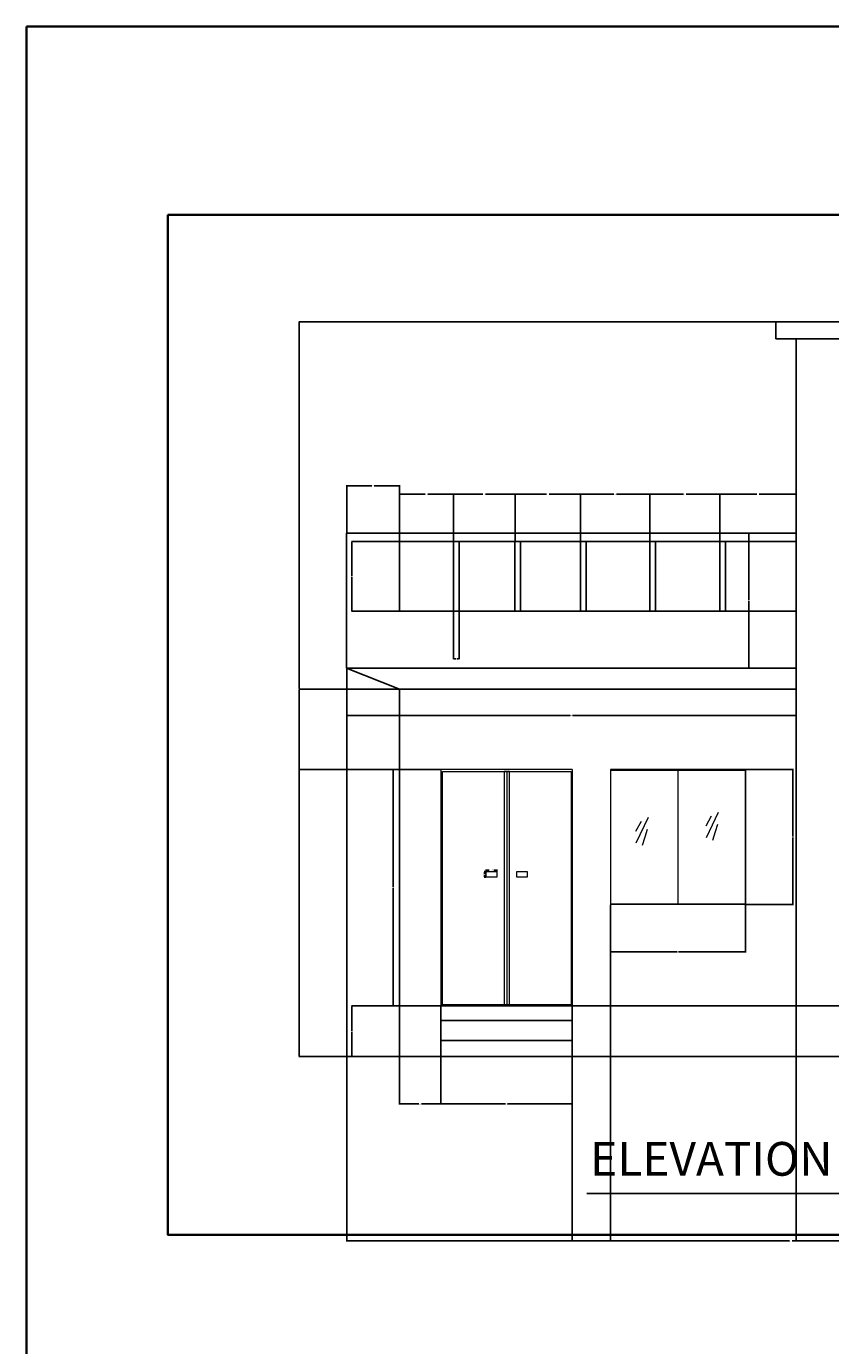
# Model space of a CAD drawing. Units: inches. Extents: x 1976 to 2558, y -977 to 2909.
# Tile 7 of 8: x 1976 to 2262, y 2441 to 2909. Entities that reach past the tile are written whole.
import ezdxf

# ---------------------------------------------------------------- set-up
doc = ezdxf.new("R2010")
doc.units = ezdxf.units.IN
for name, color, linetype, lineweight in [('A-ANNO-DIMS', 2, 'Continuous', 18), ('A-ANNO-TEXT', 7, 'Continuous', 25), ('A-ANNO-TTLB', 7, 'Continuous', 35), ('A-ELEV', 7, 'Continuous', 25), ('A-ELEV-DOOR', 3, 'Continuous', 18), ('A-ELEV-GLAZ', 4, 'Continuous', 18)]:
    doc.layers.add(name, color=color, linetype=linetype, lineweight=lineweight)
doc.styles.get("Standard").update_dxf_attribs({"font": 'arial.ttf'})
doc.dimstyles.get("Standard").update_dxf_attribs({"dimtxt": 0.18, "dimasz": 0.18, "dimexe": 0.18, "dimexo": 0.0625, "dimgap": 0.09, "dimtad": 0, "dimtih": 1, "dimtoh": 1, "dimdec": 4, "dimzin": 0, "dimdsep": 46, "dimtxsty": 'Standard', "dimcen": 0.09, "dimadec": 0, "dimazin": 0, "dimtfac": 1, "dimtdec": 4, "dimtofl": 0, "dimtmove": 0, "dimatfit": 3, "dimfxl": 1, "dimtolj": 1, "dimtzin": 0, "dimarcsym": 0})

# ---------------------------------------------------------------- blocks, each defined once
blk = doc.blocks.new('GLASS-REFLECTION')
for p, q in [((4.44, 9.97), (0.12, 0.93)), ((1.95, 8.6), (0, 5.03)), ((4.15, 5.7), (3.32, 3.04)), ((3.32, 3.04), (2.37, 0))]:
    blk.add_line(p, q)
blk = doc.blocks.new('DOOR-PULL-ELEV')
blk.add_lwpolyline([(0, 2.02), (3.74, 2.02), (3.74, 0), (0, 0)], close=True)
blk = doc.blocks.new('*D21')
at = {"layer": 'A-ANNO-DIMS', "color": 0, "lineweight": -2, "transparency": 16777216}
for p, q in [((2139.28, 2609.02), (2139.28, 2609.7)), ((2139.46, 2609.52), (2140.35, 2609.52)), ((2142.84, 2609.52), (2141.96, 2609.52)), ((2143.02, 2609.02), (2143.02, 2609.7))]:
    blk.add_line(p, q, dxfattribs=at)
at = {"layer": 'A-ANNO-DIMS', "color": 0, "transparency": 16777216}
for points in [[(2139.46, 2609.55), (2139.46, 2609.49), (2139.28, 2609.52)], [(2142.84, 2609.55), (2142.84, 2609.49), (2143.02, 2609.52)]]:
    blk.add_solid(points, dxfattribs=at)
at = {"layer": 'Defpoints', "color": 0, "transparency": 16777216}
for p in [(2139.28, 2608.96), (2143.02, 2609.52), (2143.02, 2608.96)]:
    blk.add_point(p, dxfattribs=at)
at = {"layer": 'A-ANNO-DIMS', "color": 0, "transparency": 16777216, "insert": (2141.15, 2609.52), "char_height": 0.18, "attachment_point": 5}
blk.add_mtext('\\A1;PULL 4 TYP.', dxfattribs=at)
blk = doc.blocks.new('*D22')
at = {"layer": 'A-ANNO-DIMS', "color": 0, "lineweight": -2, "transparency": 16777216}
for p, q in [((2139.22, 2608.96), (2138.54, 2608.96)), ((2139.22, 2606.94), (2138.54, 2606.94)), ((2138.72, 2608.78), (2138.72, 2608.13)), ((2138.72, 2607.12), (2138.72, 2607.77))]:
    blk.add_line(p, q, dxfattribs=at)
at = {"layer": 'A-ANNO-DIMS', "color": 0, "transparency": 16777216}
for points in [[(2138.69, 2608.78), (2138.75, 2608.78), (2138.72, 2608.96)], [(2138.69, 2607.12), (2138.75, 2607.12), (2138.72, 2606.94)]]:
    blk.add_solid(points, dxfattribs=at)
at = {"layer": 'Defpoints', "color": 0, "transparency": 16777216}
for p in [(2138.72, 2608.96), (2139.28, 2608.96), (2139.28, 2606.94)]:
    blk.add_point(p, dxfattribs=at)
at = {"layer": 'A-ANNO-DIMS', "color": 0, "transparency": 16777216, "insert": (2138.72, 2607.95), "char_height": 0.18, "attachment_point": 5}
blk.add_mtext('\\A1;2 TYP.', dxfattribs=at)
blk = doc.blocks.new('*D51')
at = {"layer": 'A-ANNO-DIMS', "color": 0, "lineweight": -2, "transparency": 16777216}
for p, q in [((2089.7, 2681.2), (2089.7, 2477.53)), ((2405.44, 2543.2), (2405.44, 2477.53)), ((2089.88, 2477.71), (2247.1, 2477.71)), ((2405.26, 2477.71), (2248.03, 2477.71))]:
    blk.add_line(p, q, dxfattribs=at)
at = {"layer": 'A-ANNO-DIMS', "color": 0, "transparency": 16777216}
for points in [[(2089.88, 2477.74), (2089.88, 2477.68), (2089.7, 2477.71)], [(2405.26, 2477.74), (2405.26, 2477.68), (2405.44, 2477.71)]]:
    blk.add_solid(points, dxfattribs=at)
at = {"layer": 'Defpoints', "color": 0, "transparency": 16777216}
for p in [(2089.7, 2681.26), (2405.44, 2543.26), (2405.44, 2477.71)]:
    blk.add_point(p, dxfattribs=at)
at = {"layer": 'A-ANNO-DIMS', "color": 0, "transparency": 16777216, "insert": (2247.57, 2477.71), "char_height": 0.18, "attachment_point": 5}
blk.add_mtext('\\A1;315.74', dxfattribs=at)
blk = doc.blocks.new('*D52')
at = {"layer": 'A-ANNO-DIMS', "color": 0, "lineweight": -2, "transparency": 16777216}
for p, q in [((2242.18, 2804.36), (2072.67, 2804.36)), ((2072.85, 2804.18), (2072.85, 2673.99)), ((2072.85, 2543.44), (2072.85, 2673.63)), ((2108.38, 2543.26), (2072.67, 2543.26))]:
    blk.add_line(p, q, dxfattribs=at)
at = {"layer": 'A-ANNO-DIMS', "color": 0, "transparency": 16777216}
for points in [[(2072.82, 2804.18), (2072.88, 2804.18), (2072.85, 2804.36)], [(2072.82, 2543.44), (2072.88, 2543.44), (2072.85, 2543.26)]]:
    blk.add_solid(points, dxfattribs=at)
at = {"layer": 'Defpoints', "color": 0, "transparency": 16777216}
for p in [(2072.85, 2804.36), (2242.24, 2804.36), (2108.44, 2543.26)]:
    blk.add_point(p, dxfattribs=at)
at = {"layer": 'A-ANNO-DIMS', "color": 0, "transparency": 16777216, "insert": (2072.85, 2673.81), "char_height": 0.18, "attachment_point": 5}
blk.add_mtext('\\A1;261.1', dxfattribs=at)
blk = doc.blocks.new('*D53')
at = {"layer": 'A-ANNO-DIMS', "color": 0, "lineweight": -2, "transparency": 16777216}
for p, q in [((2108.38, 2561.26), (2091.41, 2561.26)), ((2091.59, 2561.08), (2091.59, 2552.44)), ((2091.59, 2543.44), (2091.59, 2552.08)), ((2108.38, 2543.26), (2091.41, 2543.26))]:
    blk.add_line(p, q, dxfattribs=at)
at = {"layer": 'A-ANNO-DIMS', "color": 0, "transparency": 16777216}
for points in [[(2091.56, 2561.08), (2091.62, 2561.08), (2091.59, 2561.26)], [(2091.56, 2543.44), (2091.62, 2543.44), (2091.59, 2543.26)]]:
    blk.add_solid(points, dxfattribs=at)
at = {"layer": 'Defpoints', "color": 0, "transparency": 16777216}
for p in [(2091.59, 2561.26), (2108.44, 2561.26), (2108.44, 2543.26)]:
    blk.add_point(p, dxfattribs=at)
at = {"layer": 'A-ANNO-DIMS', "color": 0, "transparency": 16777216, "insert": (2091.59, 2552.26), "char_height": 0.18, "attachment_point": 5}
blk.add_mtext('\\A1;18', dxfattribs=at)
blk = doc.blocks.new('*D54')
at = {"layer": 'A-ANNO-DIMS', "color": 0, "lineweight": -2, "transparency": 16777216}
for p, q in [((2123.06, 2645.26), (2106.09, 2645.26)), ((2106.27, 2645.08), (2106.27, 2603.44)), ((2106.27, 2561.44), (2106.27, 2603.08)), ((2123.06, 2561.26), (2106.09, 2561.26))]:
    blk.add_line(p, q, dxfattribs=at)
at = {"layer": 'A-ANNO-DIMS', "color": 0, "transparency": 16777216}
for points in [[(2106.24, 2645.08), (2106.3, 2645.08), (2106.27, 2645.26)], [(2106.24, 2561.44), (2106.3, 2561.44), (2106.27, 2561.26)]]:
    blk.add_solid(points, dxfattribs=at)
at = {"layer": 'Defpoints', "color": 0, "transparency": 16777216}
for p in [(2106.27, 2645.26), (2123.12, 2645.26), (2123.12, 2561.26)]:
    blk.add_point(p, dxfattribs=at)
at = {"layer": 'A-ANNO-DIMS', "color": 0, "transparency": 16777216, "insert": (2106.27, 2603.26), "char_height": 0.18, "attachment_point": 5}
blk.add_mtext('\\A1;84', dxfattribs=at)
blk = doc.blocks.new('*D55')
at = {"layer": 'A-ANNO-DIMS', "color": 0, "lineweight": -2, "transparency": 16777216}
for p, q in [((2108.38, 2673.8), (2072.67, 2673.8)), ((2072.85, 2673.62), (2072.85, 2659.71)), ((2072.85, 2645.44), (2072.85, 2659.35)), ((2123.06, 2645.26), (2072.67, 2645.26))]:
    blk.add_line(p, q, dxfattribs=at)
at = {"layer": 'A-ANNO-DIMS', "color": 0, "transparency": 16777216}
for points in [[(2072.82, 2673.62), (2072.88, 2673.62), (2072.85, 2673.8)], [(2072.82, 2645.44), (2072.88, 2645.44), (2072.85, 2645.26)]]:
    blk.add_solid(points, dxfattribs=at)
at = {"layer": 'Defpoints', "color": 0, "transparency": 16777216}
for p in [(2072.85, 2673.8), (2108.44, 2673.8), (2123.12, 2645.26)]:
    blk.add_point(p, dxfattribs=at)
at = {"layer": 'A-ANNO-DIMS', "color": 0, "transparency": 16777216, "insert": (2072.85, 2659.53), "char_height": 0.18, "attachment_point": 5}
blk.add_mtext('\\A1;28.535', dxfattribs=at)
blk = doc.blocks.new('*D56')
at = {"layer": 'A-ANNO-DIMS', "color": 0, "lineweight": -2, "transparency": 16777216}
for p, q in [((2249.38, 2729.26), (2232.41, 2729.26)), ((2232.59, 2729.08), (2232.59, 2705.44)), ((2232.59, 2681.44), (2232.59, 2705.08)), ((2249.38, 2681.26), (2232.41, 2681.26))]:
    blk.add_line(p, q, dxfattribs=at)
at = {"layer": 'A-ANNO-DIMS', "color": 0, "transparency": 16777216}
for points in [[(2232.56, 2729.08), (2232.62, 2729.08), (2232.59, 2729.26)], [(2232.56, 2681.44), (2232.62, 2681.44), (2232.59, 2681.26)]]:
    blk.add_solid(points, dxfattribs=at)
at = {"layer": 'Defpoints', "color": 0, "transparency": 16777216}
for p in [(2232.59, 2729.26), (2249.44, 2729.26), (2249.44, 2681.26)]:
    blk.add_point(p, dxfattribs=at)
at = {"layer": 'A-ANNO-DIMS', "color": 0, "transparency": 16777216, "insert": (2232.59, 2705.26), "char_height": 0.18, "attachment_point": 5}
blk.add_mtext('\\A1;48', dxfattribs=at)
blk = doc.blocks.new('*D57')
at = {"layer": 'A-ANNO-DIMS', "color": 0, "lineweight": -2, "transparency": 16777216}
for p, q in [((2089.7, 2681.2), (2089.7, 2664.23)), ((2249.44, 2681.2), (2249.44, 2664.23)), ((2089.88, 2664.41), (2169.11, 2664.41)), ((2249.26, 2664.41), (2170.02, 2664.41))]:
    blk.add_line(p, q, dxfattribs=at)
at = {"layer": 'A-ANNO-DIMS', "color": 0, "transparency": 16777216}
for points in [[(2089.88, 2664.44), (2089.88, 2664.38), (2089.7, 2664.41)], [(2249.26, 2664.44), (2249.26, 2664.38), (2249.44, 2664.41)]]:
    blk.add_solid(points, dxfattribs=at)
at = {"layer": 'Defpoints', "color": 0, "transparency": 16777216}
for p in [(2089.7, 2681.26), (2249.44, 2681.26), (2089.7, 2664.41)]:
    blk.add_point(p, dxfattribs=at)
at = {"layer": 'A-ANNO-DIMS', "color": 0, "transparency": 16777216, "insert": (2169.57, 2664.41), "char_height": 0.18, "attachment_point": 5}
blk.add_mtext('\\A1;159.74', dxfattribs=at)
blk = doc.blocks.new('*D58')
at = {"layer": 'A-ANNO-DIMS', "color": 0, "lineweight": -2, "transparency": 16777216}
for p, q in [((2108.44, 2543.2), (2108.44, 2526.23)), ((2123.12, 2543.2), (2123.12, 2526.23)), ((2108.62, 2526.41), (2115.33, 2526.41)), ((2122.94, 2526.41), (2116.24, 2526.41))]:
    blk.add_line(p, q, dxfattribs=at)
at = {"layer": 'A-ANNO-DIMS', "color": 0, "transparency": 16777216}
for points in [[(2108.62, 2526.44), (2108.62, 2526.38), (2108.44, 2526.41)], [(2122.94, 2526.44), (2122.94, 2526.38), (2123.12, 2526.41)]]:
    blk.add_solid(points, dxfattribs=at)
at = {"layer": 'Defpoints', "color": 0, "transparency": 16777216}
for p in [(2108.44, 2543.26), (2123.12, 2543.26), (2108.44, 2526.41)]:
    blk.add_point(p, dxfattribs=at)
at = {"layer": 'A-ANNO-DIMS', "color": 0, "transparency": 16777216, "insert": (2115.78, 2526.41), "char_height": 0.18, "attachment_point": 5}
blk.add_mtext('\\A1;14.686', dxfattribs=at)
blk = doc.blocks.new('*D59')
at = {"layer": 'A-ANNO-DIMS', "color": 0, "lineweight": -2, "transparency": 16777216}
for p, q in [((2123.12, 2543.2), (2123.12, 2526.23)), ((2169.89, 2543.2), (2169.89, 2526.23)), ((2123.3, 2526.41), (2146.11, 2526.41)), ((2169.71, 2526.41), (2146.9, 2526.41))]:
    blk.add_line(p, q, dxfattribs=at)
at = {"layer": 'A-ANNO-DIMS', "color": 0, "transparency": 16777216}
for points in [[(2123.3, 2526.44), (2123.3, 2526.38), (2123.12, 2526.41)], [(2169.71, 2526.44), (2169.71, 2526.38), (2169.89, 2526.41)]]:
    blk.add_solid(points, dxfattribs=at)
at = {"layer": 'Defpoints', "color": 0, "transparency": 16777216}
for p in [(2123.12, 2543.26), (2169.89, 2543.26), (2123.12, 2526.41)]:
    blk.add_point(p, dxfattribs=at)
at = {"layer": 'A-ANNO-DIMS', "color": 0, "transparency": 16777216, "insert": (2146.51, 2526.41), "char_height": 0.18, "attachment_point": 5}
blk.add_mtext('\\A1;46.76', dxfattribs=at)
blk = doc.blocks.new('*D60')
at = {"layer": 'A-ANNO-DIMS', "color": 0, "lineweight": -2, "transparency": 16777216}
for p, q in [((2183.44, 2597.2), (2183.44, 2477.53)), ((2169.89, 2561.2), (2169.89, 2477.53)), ((2170.07, 2477.71), (2176.21, 2477.71)), ((2183.26, 2477.71), (2177.12, 2477.71))]:
    blk.add_line(p, q, dxfattribs=at)
at = {"layer": 'A-ANNO-DIMS', "color": 0, "transparency": 16777216}
for points in [[(2170.07, 2477.74), (2170.07, 2477.68), (2169.89, 2477.71)], [(2183.26, 2477.74), (2183.26, 2477.68), (2183.44, 2477.71)]]:
    blk.add_solid(points, dxfattribs=at)
at = {"layer": 'Defpoints', "color": 0, "transparency": 16777216}
for p in [(2183.44, 2597.26), (2169.89, 2561.26), (2183.44, 2477.71)]:
    blk.add_point(p, dxfattribs=at)
at = {"layer": 'A-ANNO-DIMS', "color": 0, "transparency": 16777216, "insert": (2176.66, 2477.71), "char_height": 0.18, "attachment_point": 5}
blk.add_mtext('\\A1;13.552', dxfattribs=at)
blk = doc.blocks.new('*D61')
at = {"layer": 'A-ANNO-DIMS', "color": 0, "lineweight": -2, "transparency": 16777216}
for p, q in [((2183.44, 2597.2), (2183.44, 2580.23)), ((2231.44, 2597.2), (2231.44, 2580.23)), ((2183.62, 2580.41), (2207.22, 2580.41)), ((2231.26, 2580.41), (2207.66, 2580.41))]:
    blk.add_line(p, q, dxfattribs=at)
at = {"layer": 'A-ANNO-DIMS', "color": 0, "transparency": 16777216}
for points in [[(2183.62, 2580.44), (2183.62, 2580.38), (2183.44, 2580.41)], [(2231.26, 2580.44), (2231.26, 2580.38), (2231.44, 2580.41)]]:
    blk.add_solid(points, dxfattribs=at)
at = {"layer": 'Defpoints', "color": 0, "transparency": 16777216}
for p in [(2183.44, 2597.26), (2231.44, 2597.26), (2183.44, 2580.41)]:
    blk.add_point(p, dxfattribs=at)
at = {"layer": 'A-ANNO-DIMS', "color": 0, "transparency": 16777216, "insert": (2207.44, 2580.41), "char_height": 0.18, "attachment_point": 5}
blk.add_mtext('\\A1;48', dxfattribs=at)
blk = doc.blocks.new('*D62')
at = {"layer": 'A-ANNO-DIMS', "color": 0, "lineweight": -2, "transparency": 16777216}
for p, q in [((2231.5, 2645.26), (2248.47, 2645.26)), ((2248.29, 2645.08), (2248.29, 2621.44)), ((2248.29, 2597.44), (2248.29, 2621.08)), ((2231.5, 2597.26), (2248.47, 2597.26))]:
    blk.add_line(p, q, dxfattribs=at)
at = {"layer": 'A-ANNO-DIMS', "color": 0, "transparency": 16777216}
for points in [[(2248.26, 2645.08), (2248.32, 2645.08), (2248.29, 2645.26)], [(2248.26, 2597.44), (2248.32, 2597.44), (2248.29, 2597.26)]]:
    blk.add_solid(points, dxfattribs=at)
at = {"layer": 'Defpoints', "color": 0, "transparency": 16777216}
for p in [(2231.44, 2645.26), (2231.44, 2597.26), (2248.29, 2597.26)]:
    blk.add_point(p, dxfattribs=at)
at = {"layer": 'A-ANNO-DIMS', "color": 0, "transparency": 16777216, "insert": (2248.29, 2621.26), "char_height": 0.18, "attachment_point": 5}
blk.add_mtext('\\A1;48', dxfattribs=at)
blk = doc.blocks.new('*D67')
at = {"layer": 'A-ANNO-DIMS', "color": 0, "lineweight": -2, "transparency": 16777216}
for p, q in [((2297.4, 2598.25), (2297.4, 2477.53)), ((2249.44, 2561.2), (2249.44, 2477.53)), ((2249.62, 2477.71), (2273.02, 2477.71)), ((2297.22, 2477.71), (2273.82, 2477.71))]:
    blk.add_line(p, q, dxfattribs=at)
at = {"layer": 'A-ANNO-DIMS', "color": 0, "transparency": 16777216}
for points in [[(2249.62, 2477.74), (2249.62, 2477.68), (2249.44, 2477.71)], [(2297.22, 2477.74), (2297.22, 2477.68), (2297.4, 2477.71)]]:
    blk.add_solid(points, dxfattribs=at)
at = {"layer": 'Defpoints', "color": 0, "transparency": 16777216}
for p in [(2297.4, 2598.31), (2249.44, 2561.26), (2249.44, 2477.71)]:
    blk.add_point(p, dxfattribs=at)
at = {"layer": 'A-ANNO-DIMS', "color": 0, "transparency": 16777216, "insert": (2273.42, 2477.71), "char_height": 0.18, "attachment_point": 5}
blk.add_mtext('\\A1;47.96', dxfattribs=at)
blk = doc.blocks.new('*D71')
at = {"layer": 'A-ANNO-DIMS', "color": 0, "lineweight": -2, "transparency": 16777216}
for p, q in [((2108.38, 2726.26), (2091.41, 2726.26)), ((2091.59, 2726.08), (2091.59, 2714.05)), ((2091.59, 2701.65), (2091.59, 2713.68)), ((2108.38, 2701.47), (2091.41, 2701.47))]:
    blk.add_line(p, q, dxfattribs=at)
at = {"layer": 'A-ANNO-DIMS', "color": 0, "transparency": 16777216}
for points in [[(2091.56, 2726.08), (2091.62, 2726.08), (2091.59, 2726.26)], [(2091.56, 2701.65), (2091.62, 2701.65), (2091.59, 2701.47)]]:
    blk.add_solid(points, dxfattribs=at)
at = {"layer": 'Defpoints', "color": 0, "transparency": 16777216}
for p in [(2091.59, 2726.26), (2108.44, 2726.26), (2108.44, 2701.47)]:
    blk.add_point(p, dxfattribs=at)
at = {"layer": 'A-ANNO-DIMS', "color": 0, "transparency": 16777216, "insert": (2091.59, 2713.87), "char_height": 0.18, "attachment_point": 5}
blk.add_mtext('\\A1;24.79', dxfattribs=at)
blk = doc.blocks.new('*D72')
at = {"layer": 'A-ANNO-DIMS', "color": 0, "lineweight": -2, "transparency": 16777216}
for p, q in [((2089.7, 2729.32), (2089.7, 2746.29)), ((2089.88, 2746.11), (2098.68, 2746.11)), ((2108.26, 2746.11), (2099.45, 2746.11)), ((2108.44, 2729.32), (2108.44, 2746.29))]:
    blk.add_line(p, q, dxfattribs=at)
at = {"layer": 'A-ANNO-DIMS', "color": 0, "transparency": 16777216}
for points in [[(2089.88, 2746.14), (2089.88, 2746.08), (2089.7, 2746.11)], [(2108.26, 2746.14), (2108.26, 2746.08), (2108.44, 2746.11)]]:
    blk.add_solid(points, dxfattribs=at)
at = {"layer": 'Defpoints', "color": 0, "transparency": 16777216}
for p in [(2108.44, 2746.11), (2089.7, 2729.26), (2108.44, 2729.26)]:
    blk.add_point(p, dxfattribs=at)
at = {"layer": 'A-ANNO-DIMS', "color": 0, "transparency": 16777216, "insert": (2099.07, 2746.11), "char_height": 0.18, "attachment_point": 5}
blk.add_mtext('\\A1;18.74', dxfattribs=at)
blk = doc.blocks.new('*D73')
at = {"layer": 'A-ANNO-DIMS', "color": 0, "lineweight": -2, "transparency": 16777216}
for p, q in [((2108.44, 2726.32), (2108.44, 2743.29)), ((2108.62, 2743.11), (2117.6, 2743.11)), ((2127.48, 2743.11), (2118.51, 2743.11)), ((2127.66, 2726.32), (2127.66, 2743.29))]:
    blk.add_line(p, q, dxfattribs=at)
at = {"layer": 'A-ANNO-DIMS', "color": 0, "transparency": 16777216}
for points in [[(2108.62, 2743.14), (2108.62, 2743.08), (2108.44, 2743.11)], [(2127.48, 2743.14), (2127.48, 2743.08), (2127.66, 2743.11)]]:
    blk.add_solid(points, dxfattribs=at)
at = {"layer": 'Defpoints', "color": 0, "transparency": 16777216}
for p in [(2127.66, 2743.11), (2108.44, 2726.26), (2127.66, 2726.26)]:
    blk.add_point(p, dxfattribs=at)
at = {"layer": 'A-ANNO-DIMS', "color": 0, "transparency": 16777216, "insert": (2118.05, 2743.11), "char_height": 0.18, "attachment_point": 5}
blk.add_mtext('\\A1;19.224', dxfattribs=at)
blk = doc.blocks.new('*D74')
at = {"layer": 'A-ANNO-DIMS', "color": 0, "lineweight": -2, "transparency": 16777216}
for p, q in [((2127.66, 2726.32), (2127.66, 2743.29)), ((2127.84, 2743.11), (2138.13, 2743.11)), ((2149.35, 2743.11), (2139.06, 2743.11)), ((2149.53, 2726.32), (2149.53, 2743.29))]:
    blk.add_line(p, q, dxfattribs=at)
at = {"layer": 'A-ANNO-DIMS', "color": 0, "transparency": 16777216}
for points in [[(2127.84, 2743.14), (2127.84, 2743.08), (2127.66, 2743.11)], [(2149.35, 2743.14), (2149.35, 2743.08), (2149.53, 2743.11)]]:
    blk.add_solid(points, dxfattribs=at)
at = {"layer": 'Defpoints', "color": 0, "transparency": 16777216}
for p in [(2149.53, 2743.11), (2127.66, 2726.26), (2149.53, 2726.26)]:
    blk.add_point(p, dxfattribs=at)
at = {"layer": 'A-ANNO-DIMS', "color": 0, "transparency": 16777216, "insert": (2138.6, 2743.11), "char_height": 0.18, "attachment_point": 5}
blk.add_mtext('\\A1;21.866', dxfattribs=at)
blk = doc.blocks.new('*D75')
at = {"layer": 'A-ANNO-DIMS', "color": 0, "lineweight": -2, "transparency": 16777216}
for p, q in [((2149.53, 2726.32), (2149.53, 2743.29)), ((2149.71, 2743.11), (2160.69, 2743.11)), ((2172.61, 2743.11), (2161.62, 2743.11)), ((2172.79, 2726.32), (2172.79, 2743.29))]:
    blk.add_line(p, q, dxfattribs=at)
at = {"layer": 'A-ANNO-DIMS', "color": 0, "transparency": 16777216}
for points in [[(2149.71, 2743.14), (2149.71, 2743.08), (2149.53, 2743.11)], [(2172.61, 2743.14), (2172.61, 2743.08), (2172.79, 2743.11)]]:
    blk.add_solid(points, dxfattribs=at)
at = {"layer": 'Defpoints', "color": 0, "transparency": 16777216}
for p in [(2172.79, 2743.11), (2149.53, 2726.26), (2172.79, 2726.26)]:
    blk.add_point(p, dxfattribs=at)
at = {"layer": 'A-ANNO-DIMS', "color": 0, "transparency": 16777216, "insert": (2161.16, 2743.11), "char_height": 0.18, "attachment_point": 5}
blk.add_mtext('\\A1;23.263', dxfattribs=at)
blk = doc.blocks.new('*D76')
at = {"layer": 'A-ANNO-DIMS', "color": 0, "lineweight": -2, "transparency": 16777216}
for p, q in [((2172.79, 2726.32), (2172.79, 2743.29)), ((2172.97, 2743.11), (2184.65, 2743.11)), ((2197.26, 2743.11), (2185.58, 2743.11)), ((2197.44, 2726.32), (2197.44, 2743.29))]:
    blk.add_line(p, q, dxfattribs=at)
at = {"layer": 'A-ANNO-DIMS', "color": 0, "transparency": 16777216}
for points in [[(2172.97, 2743.14), (2172.97, 2743.08), (2172.79, 2743.11)], [(2197.26, 2743.14), (2197.26, 2743.08), (2197.44, 2743.11)]]:
    blk.add_solid(points, dxfattribs=at)
at = {"layer": 'Defpoints', "color": 0, "transparency": 16777216}
for p in [(2197.44, 2743.11), (2172.79, 2726.26), (2197.44, 2726.26)]:
    blk.add_point(p, dxfattribs=at)
at = {"layer": 'A-ANNO-DIMS', "color": 0, "transparency": 16777216, "insert": (2185.11, 2743.11), "char_height": 0.18, "attachment_point": 5}
blk.add_mtext('\\A1;24.646', dxfattribs=at)
blk = doc.blocks.new('*D77')
at = {"layer": 'A-ANNO-DIMS', "color": 0, "lineweight": -2, "transparency": 16777216}
for p, q in [((2197.44, 2726.32), (2197.44, 2743.29)), ((2197.62, 2743.11), (2209.41, 2743.11)), ((2222.14, 2743.11), (2210.34, 2743.11)), ((2222.32, 2726.32), (2222.32, 2743.29))]:
    blk.add_line(p, q, dxfattribs=at)
at = {"layer": 'A-ANNO-DIMS', "color": 0, "transparency": 16777216}
for points in [[(2197.62, 2743.14), (2197.62, 2743.08), (2197.44, 2743.11)], [(2222.14, 2743.14), (2222.14, 2743.08), (2222.32, 2743.11)]]:
    blk.add_solid(points, dxfattribs=at)
at = {"layer": 'Defpoints', "color": 0, "transparency": 16777216}
for p in [(2222.32, 2743.11), (2197.44, 2726.26), (2222.32, 2726.26)]:
    blk.add_point(p, dxfattribs=at)
at = {"layer": 'A-ANNO-DIMS', "color": 0, "transparency": 16777216, "insert": (2209.88, 2743.11), "char_height": 0.18, "attachment_point": 5}
blk.add_mtext('\\A1;24.884', dxfattribs=at)
blk = doc.blocks.new('*D78')
at = {"layer": 'A-ANNO-DIMS', "color": 0, "lineweight": -2, "transparency": 16777216}
for p, q in [((2222.32, 2726.32), (2222.32, 2743.29)), ((2222.5, 2743.11), (2235.49, 2743.11)), ((2249.26, 2743.11), (2236.27, 2743.11)), ((2249.44, 2726.32), (2249.44, 2743.29))]:
    blk.add_line(p, q, dxfattribs=at)
at = {"layer": 'A-ANNO-DIMS', "color": 0, "transparency": 16777216}
for points in [[(2222.5, 2743.14), (2222.5, 2743.08), (2222.32, 2743.11)], [(2249.26, 2743.14), (2249.26, 2743.08), (2249.44, 2743.11)]]:
    blk.add_solid(points, dxfattribs=at)
at = {"layer": 'Defpoints', "color": 0, "transparency": 16777216}
for p in [(2249.44, 2743.11), (2222.32, 2726.26), (2249.44, 2726.26)]:
    blk.add_point(p, dxfattribs=at)
at = {"layer": 'A-ANNO-DIMS', "color": 0, "transparency": 16777216, "insert": (2235.88, 2743.11), "char_height": 0.18, "attachment_point": 5}
blk.add_mtext('\\A1;27.12', dxfattribs=at)
blk = doc.blocks.new('*D79')
at = {"layer": 'A-ANNO-DIMS', "color": 0, "lineweight": -2, "transparency": 16777216}
for p, q in [((2127.66, 2701.41), (2127.66, 2684.44)), ((2129.66, 2701.41), (2129.66, 2684.44)), ((2127.84, 2684.62), (2128.51, 2684.62)), ((2129.48, 2684.62), (2128.81, 2684.62))]:
    blk.add_line(p, q, dxfattribs=at)
at = {"layer": 'A-ANNO-DIMS', "color": 0, "transparency": 16777216}
for points in [[(2127.84, 2684.65), (2127.84, 2684.59), (2127.66, 2684.62)], [(2129.48, 2684.65), (2129.48, 2684.59), (2129.66, 2684.62)]]:
    blk.add_solid(points, dxfattribs=at)
at = {"layer": 'Defpoints', "color": 0, "transparency": 16777216}
for p in [(2127.66, 2701.47), (2129.66, 2701.47), (2127.66, 2684.62)]:
    blk.add_point(p, dxfattribs=at)
at = {"layer": 'A-ANNO-DIMS', "color": 0, "transparency": 16777216, "insert": (2128.66, 2684.62), "char_height": 0.18, "attachment_point": 5}
blk.add_mtext('\\A1;2', dxfattribs=at)

msp = doc.modelspace()

# ---------------------------------------------------------------- linework, layer by layer
at = {"layer": 'A-ANNO-TEXT'}
msp.add_line((2175.0551, 2494.5563), (2270.2236, 2494.5563), dxfattribs=at)
at = {"layer": 'A-ANNO-TTLB'}
for points in [[(1975.8545, 2909.3429), (2557.9168, 2909.3429), (2557.9168, 1747.8598), (1975.8545, 1747.8598)], [(2026.154, 2842.3802), (2486.7724, 2842.3802), (2486.7724, 2479.8768), (2026.154, 2479.8768)]]:
    msp.add_lwpolyline(points, close=True, dxfattribs=at)
at = {"layer": 'A-ELEV'}
for p, q in [((2405.4385, 2804.3628), (2242.2431, 2804.3628)), ((2242.2431, 2804.3628), (2242.2431, 2798.3628)), ((2242.2431, 2798.3628), (2405.4385, 2798.3628)), ((2249.4385, 2729.2601), (2249.4385, 2798.3628)), ((2089.697, 2681.2601), (2089.697, 2729.2601)), ((2089.697, 2729.2601), (2108.4385, 2729.2601)), ((2089.697, 2729.2601), (2089.697, 2726.2601)), ((2249.4385, 2729.2601), (2108.4385, 2729.2601)), ((2108.4385, 2729.2601), (2108.4385, 2701.4709)), ((2249.4385, 2681.2601), (2249.4385, 2729.2601)), ((2108.4385, 2726.2601), (2249.4385, 2726.2601)), ((2127.6621, 2726.2601), (2127.6621, 2701.4709)), ((2129.6621, 2701.4709), (2129.6621, 2726.2601)), ((2149.5281, 2726.2601), (2149.5281, 2701.4709)), ((2151.5281, 2701.4709), (2151.5281, 2726.2601)), ((2172.7909, 2726.2601), (2172.7909, 2701.4709)), ((2174.7909, 2701.4709), (2174.7909, 2726.2601)), ((2197.4365, 2726.2601), (2197.4365, 2701.4709)), ((2199.4365, 2701.4709), (2199.4365, 2726.2601)), ((2222.3202, 2726.2601), (2222.3202, 2701.4709)), ((2224.3202, 2701.4709), (2224.3202, 2726.2601)), ((2108.4385, 2701.4709), (2249.4385, 2701.4709)), ((2127.6621, 2701.4709), (2129.6621, 2701.4709)), ((2108.4385, 2681.2601), (2089.697, 2681.2601)), ((2089.697, 2681.2601), (2108.4385, 2673.795)), ((2249.4385, 2681.2601), (2108.4385, 2681.2601)), ((2249.4385, 2681.2601), (2249.4385, 2561.2601)), ((2108.4385, 2673.795), (2108.4385, 2543.2601)), ((2108.4385, 2673.795), (2249.4385, 2673.795)), ((2405.4385, 2561.2601), (2108.4385, 2561.2601)), ((2123.1248, 2561.2601), (2123.1248, 2543.2601)), ((2169.8866, 2561.2601), (2169.8866, 2543.2601)), ((2123.1248, 2556.0879), (2169.8866, 2556.0879)), ((2123.1248, 2548.9576), (2169.8866, 2548.9576)), ((2405.4385, 2543.2601), (2108.4385, 2543.2601))]:
    msp.add_line(p, q, dxfattribs=at)
at = {"layer": 'A-ELEV-DOOR'}
for p, q in [((2169.8866, 2645.2601), (2123.1248, 2645.2601)), ((2169.8866, 2645.2601), (2123.1248, 2645.2601)), ((2123.1248, 2645.2601), (2123.1248, 2561.2601)), ((2146.6233, 2644.5191), (2145.6233, 2644.5191)), ((2145.6233, 2644.5191), (2145.6233, 2561.5892)), ((2146.6233, 2644.5191), (2146.6233, 2561.5892)), ((2147.6233, 2644.5191), (2146.6233, 2644.5191)), ((2147.6233, 2561.5892), (2147.6233, 2644.5191)), ((2169.8866, 2645.2601), (2169.8866, 2561.2601)), ((2146.6233, 2561.5892), (2147.6233, 2561.5892))]:
    msp.add_line(p, q, dxfattribs=at)
msp.add_lwpolyline([(2123.7768, 2644.5191), (2169.4699, 2644.5191), (2169.4699, 2561.5892), (2123.7768, 2561.5892)], close=True, dxfattribs=at)
at = {"layer": 'A-ELEV-GLAZ'}
for p, q in [((2183.4385, 2645.2601), (2183.4385, 2597.2601)), ((2231.4385, 2645.2601), (2183.4385, 2645.2601)), ((2231.4385, 2645.2601), (2183.4385, 2645.2601)), ((2207.4626, 2645.0642), (2207.4626, 2597.4154)), ((2231.4385, 2645.2601), (2231.4385, 2597.2601)), ((2231.4385, 2597.2601), (2183.4385, 2597.2601))]:
    msp.add_line(p, q, dxfattribs=at)
msp.add_lwpolyline([(2183.6256, 2645.0642), (2231.2997, 2645.0642), (2231.2997, 2597.4154), (2183.6256, 2597.4154)], close=True, dxfattribs=at)

# ---------------------------------------------------------------- block references
at = {"layer": 'A-ELEV-DOOR'}
for p in [(2139.2833, 2606.939), (2150.159, 2606.939)]:
    msp.add_blockref('DOOR-PULL-ELEV', p, dxfattribs=at)
at = {"layer": 'A-ELEV-GLAZ'}
for p in [(2192.397, 2618.2007), (2217.333, 2620.067)]:
    msp.add_blockref('GLASS-REFLECTION', p, dxfattribs=at)

# ---------------------------------------------------------------- texts
at = {"layer": 'A-ANNO-TEXT', "insert": (2176.248, 2512.8969), "char_height": 12, "attachment_point": 1}
msp.add_mtext_dynamic_manual_height_columns('ELEVATION', width=191.481289, gutter_width=12.5, heights=[0], dxfattribs=at)

# ---------------------------------------------------------------- dimensions: what is measured, and where the dimension line sits
at = {"layer": 'A-ANNO-DIMS'}
for base, p1, p2, angle, override, picture, middle in [((2072.847, 2804.3628), (2108.4385, 2543.2601), (2242.2431, 2804.3628), 90, {"dimdec": 1, "dimlfac": 1, "dimrnd": 0, "dimzin": 0, "dimdsep": 46, "dimlunit": 2}, '*D52', (2072.847, 2673.8114)), ((2127.6621, 2743.1101), (2108.4385, 2726.2601), (2127.6621, 2726.2601), 0, {"dimdec": 3, "dimlfac": 1, "dimrnd": 0, "dimzin": 0, "dimdsep": 46, "dimlunit": 2}, '*D73', (2118.0503, 2743.1101)), ((2197.4365, 2743.1101), (2172.7909, 2726.2601), (2197.4365, 2726.2601), 0, {"dimdec": 3, "dimlfac": 1, "dimrnd": 0, "dimzin": 0, "dimdsep": 46, "dimlunit": 2}, '*D76', (2185.1137, 2743.1101)), ((2232.5885, 2729.2601), (2249.4385, 2681.2601), (2249.4385, 2729.2601), 90, {"dimdec": 0, "dimlfac": 1, "dimrnd": 0, "dimzin": 0, "dimdsep": 46, "dimlunit": 2}, '*D56', (2232.5885, 2705.2601)), ((2091.5885, 2726.2601), (2108.4385, 2701.4709), (2108.4385, 2726.2601), 90, {"dimdec": 2, "dimlfac": 1, "dimrnd": 0, "dimzin": 0, "dimdsep": 46, "dimlunit": 2}, '*D71', (2091.5885, 2713.8655)), ((2127.6621, 2684.6209), (2129.6621, 2701.4709), (2127.6621, 2701.4709), 180, {"dimdec": 0, "dimlfac": 1, "dimrnd": 0, "dimzin": 0, "dimdsep": 46, "dimlunit": 2}, '*D79', (2128.6621, 2684.6209)), ((2089.697, 2664.4101), (2249.4385, 2681.2601), (2089.697, 2681.2601), 180, {"dimdec": 2, "dimlfac": 1, "dimrnd": 0, "dimzin": 0, "dimdsep": 46, "dimlunit": 2}, '*D57', (2169.5677, 2664.4101)), ((2072.847, 2673.795), (2123.1248, 2645.2601), (2108.4385, 2673.795), 90, {"dimdec": 3, "dimlfac": 1, "dimrnd": 0, "dimzin": 0, "dimdsep": 46, "dimlunit": 2}, '*D55', (2072.847, 2659.5275)), ((2106.2748, 2645.2601), (2123.1248, 2561.2601), (2123.1248, 2645.2601), 90, {"dimdec": 0, "dimlfac": 1, "dimrnd": 0, "dimzin": 0, "dimdsep": 46, "dimlunit": 2}, '*D54', (2106.2748, 2603.2601)), ((2248.2885, 2597.2601), (2231.4385, 2645.2601), (2231.4385, 2597.2601), 270, {"dimdec": 0, "dimlfac": 1, "dimrnd": 0, "dimzin": 0, "dimdsep": 46, "dimlunit": 2}, '*D62', (2248.2885, 2621.2601)), ((2183.4385, 2580.4101), (2231.4385, 2597.2601), (2183.4385, 2597.2601), 180, {"dimdec": 0, "dimlfac": 1, "dimrnd": 0, "dimzin": 0, "dimdsep": 46, "dimlunit": 2}, '*D61', (2207.4385, 2580.4101)), ((2091.5885, 2561.2601), (2108.4385, 2543.2601), (2108.4385, 2561.2601), 90, {"dimdec": 0, "dimlfac": 1, "dimrnd": 0, "dimzin": 0, "dimdsep": 46, "dimlunit": 2}, '*D53', (2091.5885, 2552.2601)), ((2108.4385, 2526.4101), (2123.1248, 2543.2601), (2108.4385, 2543.2601), 180, {"dimdec": 3, "dimlfac": 1, "dimrnd": 0, "dimzin": 0, "dimdsep": 46, "dimlunit": 2}, '*D58', (2115.7816, 2526.4101)), ((2123.1248, 2526.4101), (2169.8866, 2543.2601), (2123.1248, 2543.2601), 180, {"dimdec": 2, "dimlfac": 1, "dimrnd": 0, "dimzin": 0, "dimdsep": 46, "dimlunit": 2}, '*D59', (2146.5057, 2526.4101))]:
    dim = msp.add_linear_dim(base=base, p1=p1, p2=p2, angle=angle, dimstyle='Standard', override=override, dxfattribs=at)
    dim.commit()
    dim.dimension.update_dxf_attribs({"geometry": picture, "text_midpoint": middle})
for base, p1, p2, override, picture, middle in [((2108.4385, 2746.1101), (2089.697, 2729.2601), (2108.4385, 2729.2601), {"dimdec": 2, "dimlfac": 1, "dimrnd": 0, "dimzin": 0, "dimdsep": 46, "dimlunit": 2}, '*D72', (2099.0677, 2746.1101)), ((2149.5281, 2743.1101), (2127.6621, 2726.2601), (2149.5281, 2726.2601), {"dimdec": 3, "dimlfac": 1, "dimrnd": 0, "dimzin": 0, "dimdsep": 46, "dimlunit": 2}, '*D74', (2138.5951, 2743.1101)), ((2172.7909, 2743.1101), (2149.5281, 2726.2601), (2172.7909, 2726.2601), {"dimdec": 3, "dimlfac": 1, "dimrnd": 0, "dimzin": 0, "dimdsep": 46, "dimlunit": 2}, '*D75', (2161.1595, 2743.1101)), ((2222.3202, 2743.1101), (2197.4365, 2726.2601), (2222.3202, 2726.2601), {"dimdec": 3, "dimlfac": 1, "dimrnd": 0, "dimzin": 0, "dimdsep": 46, "dimlunit": 2}, '*D77', (2209.8783, 2743.1101)), ((2249.4385, 2743.1101), (2222.3202, 2726.2601), (2249.4385, 2726.2601), {"dimdec": 2, "dimlfac": 1, "dimrnd": 0, "dimzin": 0, "dimdsep": 46, "dimlunit": 2}, '*D78', (2235.8793, 2743.1101)), ((2405.4385, 2477.7063), (2089.697, 2681.2601), (2405.4385, 2543.2601), {"dimdec": 2, "dimlfac": 1, "dimrnd": 0, "dimzin": 0, "dimdsep": 46, "dimlunit": 2}, '*D51', (2247.5677, 2477.7063)), ((2183.4385, 2477.7063), (2169.8866, 2561.2601), (2183.4385, 2597.2601), {"dimdec": 3, "dimlfac": 1, "dimrnd": 0, "dimzin": 0, "dimdsep": 46, "dimlunit": 2}, '*D60', (2176.6625, 2477.7063)), ((2249.4385, 2477.7063), (2297.4015, 2598.3119), (2249.4385, 2561.2601), {"dimdec": 2, "dimlfac": 1, "dimrnd": 0, "dimzin": 0, "dimdsep": 46, "dimlunit": 2}, '*D67', (2273.42, 2477.7063))]:
    dim = msp.add_linear_dim(base=base, p1=p1, p2=p2, dimstyle='Standard', override=override, dxfattribs=at)
    dim.commit()
    dim.dimension.update_dxf_attribs({"geometry": picture, "text_midpoint": middle})
dim = msp.add_linear_dim(base=(2138.7218, 2608.9622), p1=(2139.2829, 2606.9392), p2=(2139.2829, 2608.9622), angle=90, text='<> TYP.', dimstyle='Standard', override={"dimdec": 0, "dimlfac": 1, "dimrnd": 0, "dimzin": 0, "dimdsep": 46, "dimlunit": 2}, dxfattribs=at)
dim.commit()
dim.dimension.update_dxf_attribs({"geometry": '*D22', "text_midpoint": (2138.7218, 2607.9507)})
dim = msp.add_linear_dim(base=(2143.0239, 2609.5233), p1=(2139.2829, 2608.9622), p2=(2143.0239, 2608.9622), text='PULL <> TYP.', dimstyle='Standard', override={"dimdec": 0, "dimlfac": 1, "dimrnd": 0, "dimzin": 0, "dimdsep": 46, "dimlunit": 2}, dxfattribs=at)
dim.commit()
dim.dimension.update_dxf_attribs({"geometry": '*D21', "text_midpoint": (2141.1534, 2609.5233)})

doc.saveas('drawing.dxf')
